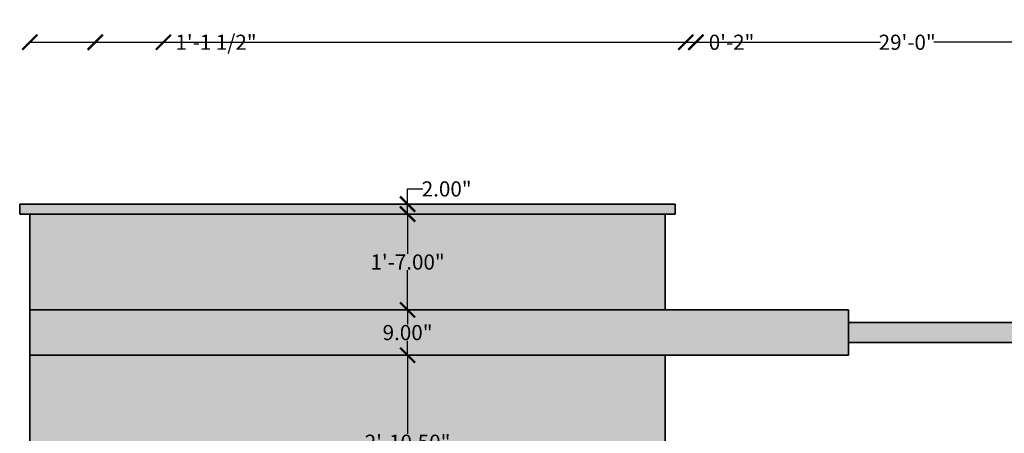
# Model space of a CAD drawing. Units: inches. Extents: x -654 to 390, y -40 to 648.
# Tile 12 of 13: x -3 to 192, y 566 to 648. Entities that reach past the tile are written whole.
import ezdxf

# ---------------------------------------------------------------- set-up
doc = ezdxf.new("R2010")
doc.units = ezdxf.units.IN
doc.header["$PDMODE"] = 3
for name, color, linetype, lineweight in [('A-ANNO-DIMS', 2, 'Continuous', 18), ('A-ELEV', 7, 'Continuous', 35), ('A-ELEV-FILL', 252, 'Continuous', 13)]:
    doc.layers.add(name, color=color, linetype=linetype, lineweight=lineweight)
doc.styles.get("Standard").update_dxf_attribs({"font": 'arial.ttf'})
doc.dimstyles.get("Standard").update_dxf_attribs({"dimtxt": 3, "dimasz": 3, "dimexe": 0.18, "dimexo": 0.0625, "dimgap": 0.09, "dimtad": 0, "dimtih": 1, "dimtoh": 1, "dimzin": 0, "dimdsep": 46, "dimlunit": 3, "dimtxsty": 'Standard', "dimblk": 'ARCHTICK', "dimcen": 0.09, "dimse1": 1, "dimse2": 1, "dimadec": 0, "dimazin": 0, "dimtfac": 1, "dimtofl": 0, "dimtmove": 0, "dimatfit": 3, "dimfxl": 1, "dimtolj": 1, "dimtzin": 0, "dimarcsym": 0})

# ---------------------------------------------------------------- blocks, each defined once
blk = doc.blocks.new('_ArchTick')
at = {"color": 0, "linetype": 'ByBlock', "const_width": 0.15}
blk.add_lwpolyline([(-0.5, -0.5), (0.5, 0.5)], dxfattribs=at)
blk = doc.blocks.new('*D8')
at = {"layer": 'A-ANNO-DIMS', "color": 0, "lineweight": -2, "transparency": 16777216}
for p, q in [((360.51, 590.13), (360.51, 545.26)), ((360.51, 497.13), (360.51, 542.01))]:
    blk.add_line(p, q, dxfattribs=at)
at = {"layer": 'Defpoints', "color": 0, "transparency": 16777216}
for p in [(161.04, 590.13), (360.51, 590.13), (346.65, 497.13)]:
    blk.add_point(p, dxfattribs=at)
at = {"layer": 'A-ANNO-DIMS', "color": 0, "lineweight": -2, "transparency": 16777216, "xscale": 3, "yscale": 3, "zscale": 3}
for p, rotation in [((360.51, 590.13), 90), ((360.51, 497.13), 270)]:
    blk.add_blockref('_ArchTick', p, dxfattribs=dict(at, rotation=rotation))
at = {"layer": 'A-ANNO-DIMS', "color": 0, "transparency": 16777216, "insert": (360.51, 543.63), "char_height": 3, "attachment_point": 5}
blk.add_mtext('\\A1;7\'-9.00"', dxfattribs=at)
blk = doc.blocks.new('*D9')
at = {"layer": 'A-ANNO-DIMS', "color": 0, "lineweight": -2, "transparency": 16777216}
for p, q in [((360.51, 611.13), (360.51, 602.26)), ((360.51, 590.13), (360.51, 599.01))]:
    blk.add_line(p, q, dxfattribs=at)
at = {"layer": 'Defpoints', "color": 0, "transparency": 16777216}
for p in [(126.65, 611.13), (360.51, 611.13), (161.04, 590.13)]:
    blk.add_point(p, dxfattribs=at)
at = {"layer": 'A-ANNO-DIMS', "color": 0, "lineweight": -2, "transparency": 16777216, "xscale": 3, "yscale": 3, "zscale": 3}
for p, rotation in [((360.51, 611.13), 90), ((360.51, 590.13), 270)]:
    blk.add_blockref('_ArchTick', p, dxfattribs=dict(at, rotation=rotation))
at = {"layer": 'A-ANNO-DIMS', "color": 0, "transparency": 16777216, "insert": (360.51, 600.63), "char_height": 3, "attachment_point": 5}
blk.add_mtext('\\A1;1\'-9.00"', dxfattribs=at)
blk = doc.blocks.new('*D10')
at = {"layer": 'A-ANNO-DIMS', "color": 0, "lineweight": -2, "transparency": 16777216}
for p, q in [((73.57, 611.13), (73.57, 614.13)), ((73.57, 614.13), (76.57, 614.13)), ((73.57, 609.13), (73.57, 611.13))]:
    blk.add_line(p, q, dxfattribs=at)
at = {"layer": 'Defpoints', "color": 0, "transparency": 16777216}
for p in [(61.65, 611.13), (73.57, 611.13), (61.65, 609.13)]:
    blk.add_point(p, dxfattribs=at)
at = {"layer": 'A-ANNO-DIMS', "color": 0, "lineweight": -2, "transparency": 16777216, "xscale": 3, "yscale": 3, "zscale": 3}
for p, rotation in [((73.57, 611.13), 90), ((73.57, 609.13), 270)]:
    blk.add_blockref('_ArchTick', p, dxfattribs=dict(at, rotation=rotation))
at = {"layer": 'A-ANNO-DIMS', "color": 0, "transparency": 16777216, "insert": (81.32, 614.13), "char_height": 3, "attachment_point": 5}
blk.add_mtext('\\A1;2.00"', dxfattribs=at)
blk = doc.blocks.new('*D11')
at = {"layer": 'A-ANNO-DIMS', "color": 0, "lineweight": -2, "transparency": 16777216}
for p, q in [((73.57, 609.13), (73.57, 601.26)), ((73.57, 590.13), (73.57, 598.01))]:
    blk.add_line(p, q, dxfattribs=at)
at = {"layer": 'Defpoints', "color": 0, "transparency": 16777216}
for p in [(73.57, 609.13), (73.57, 590.13), (73.57, 590.13)]:
    blk.add_point(p, dxfattribs=at)
at = {"layer": 'A-ANNO-DIMS', "color": 0, "lineweight": -2, "transparency": 16777216, "xscale": 3, "yscale": 3, "zscale": 3}
for p, rotation in [((73.57, 609.13), 90), ((73.57, 590.13), 270)]:
    blk.add_blockref('_ArchTick', p, dxfattribs=dict(at, rotation=rotation))
at = {"layer": 'A-ANNO-DIMS', "color": 0, "transparency": 16777216, "insert": (73.57, 599.63), "char_height": 3, "attachment_point": 5}
blk.add_mtext('\\A1;1\'-7.00"', dxfattribs=at)
blk = doc.blocks.new('*D12')
at = {"layer": 'A-ANNO-DIMS', "color": 0, "lineweight": -2, "transparency": 16777216}
for p, q in [((73.57, 590.13), (73.57, 587.26)), ((73.57, 581.13), (73.57, 584.01))]:
    blk.add_line(p, q, dxfattribs=at)
at = {"layer": 'Defpoints', "color": 0, "transparency": 16777216}
for p in [(73.57, 590.13), (73.57, 581.13), (73.57, 581.13)]:
    blk.add_point(p, dxfattribs=at)
at = {"layer": 'A-ANNO-DIMS', "color": 0, "lineweight": -2, "transparency": 16777216, "xscale": 3, "yscale": 3, "zscale": 3}
for p, rotation in [((73.57, 590.13), 90), ((73.57, 581.13), 270)]:
    blk.add_blockref('_ArchTick', p, dxfattribs=dict(at, rotation=rotation))
at = {"layer": 'A-ANNO-DIMS', "color": 0, "transparency": 16777216, "insert": (73.57, 585.63), "char_height": 3, "attachment_point": 5}
blk.add_mtext('\\A1;9.00"', dxfattribs=at)
blk = doc.blocks.new('*D13')
at = {"layer": 'A-ANNO-DIMS', "color": 0, "lineweight": -2, "transparency": 16777216}
for p, q in [((73.57, 581.13), (73.57, 565.51)), ((73.57, 546.63), (73.57, 562.26))]:
    blk.add_line(p, q, dxfattribs=at)
at = {"layer": 'Defpoints', "color": 0, "transparency": 16777216}
for p in [(73.57, 581.13), (57.15, 546.63), (73.57, 546.63)]:
    blk.add_point(p, dxfattribs=at)
at = {"layer": 'A-ANNO-DIMS', "color": 0, "lineweight": -2, "transparency": 16777216, "xscale": 3, "yscale": 3, "zscale": 3}
for p, rotation in [((73.57, 581.13), 90), ((73.57, 546.63), 270)]:
    blk.add_blockref('_ArchTick', p, dxfattribs=dict(at, rotation=rotation))
at = {"layer": 'A-ANNO-DIMS', "color": 0, "transparency": 16777216, "insert": (73.57, 563.88), "char_height": 3, "attachment_point": 5}
blk.add_mtext('\\A1;2\'-10.50"', dxfattribs=at)
blk = doc.blocks.new('*D75')
at = {"layer": 'A-ANNO-DIMS', "color": 0, "lineweight": -2, "transparency": 16777216}
for p, q in [((-1.35, 643.23), (167.38, 643.23)), ((346.65, 643.23), (177.91, 643.23))]:
    blk.add_line(p, q, dxfattribs=at)
at = {"layer": 'Defpoints', "color": 0, "transparency": 16777216}
for p in [(346.65, 643.23), (-1.35, 611.13), (346.65, 587.63)]:
    blk.add_point(p, dxfattribs=at)
at = {"layer": 'A-ANNO-DIMS', "color": 0, "lineweight": -2, "transparency": 16777216, "xscale": 3, "yscale": 3, "zscale": 3, "rotation": 180}
blk.add_blockref('_ArchTick', (-1.35, 643.23), dxfattribs=at)
at = {"layer": 'A-ANNO-DIMS', "color": 0, "lineweight": -2, "transparency": 16777216, "xscale": 3, "yscale": 3, "zscale": 3}
blk.add_blockref('_ArchTick', (346.65, 643.23), dxfattribs=at)
at = {"layer": 'A-ANNO-DIMS', "color": 0, "transparency": 16777216, "insert": (172.65, 643.23), "char_height": 3, "attachment_point": 5}
blk.add_mtext('\\A1;29\'-0"', dxfattribs=at)
blk = doc.blocks.new('*D76')
at = {"layer": 'A-ANNO-DIMS', "color": 0, "lineweight": -2, "transparency": 16777216}
for p, q in [((380.75, 611.13), (380.75, 306.76)), ((380.75, -0.87), (380.75, 303.51))]:
    blk.add_line(p, q, dxfattribs=at)
at = {"layer": 'Defpoints', "color": 0, "transparency": 16777216}
for p in [(126.65, 611.13), (380.75, 611.13), (346.65, -0.87)]:
    blk.add_point(p, dxfattribs=at)
at = {"layer": 'A-ANNO-DIMS', "color": 0, "lineweight": -2, "transparency": 16777216, "xscale": 3, "yscale": 3, "zscale": 3}
for p, rotation in [((380.75, 611.13), 90), ((380.75, -0.87), 270)]:
    blk.add_blockref('_ArchTick', p, dxfattribs=dict(at, rotation=rotation))
at = {"layer": 'A-ANNO-DIMS', "color": 0, "transparency": 16777216, "insert": (380.75, 305.13), "char_height": 3, "attachment_point": 5}
blk.add_mtext('\\A1;51\'-0"', dxfattribs=at)
blk = doc.blocks.new('*D80')
at = {"layer": 'A-ANNO-DIMS', "color": 0, "lineweight": -2, "transparency": 16777216}
for p, q in [((11.65, 643.23), (25.15, 643.23)), ((25.15, 643.23), (28.15, 643.23))]:
    blk.add_line(p, q, dxfattribs=at)
at = {"layer": 'Defpoints', "color": 0, "transparency": 16777216}
for p in [(25.15, 643.23), (11.65, 20.08), (25.15, 20.08)]:
    blk.add_point(p, dxfattribs=at)
at = {"layer": 'A-ANNO-DIMS', "color": 0, "lineweight": -2, "transparency": 16777216, "xscale": 3, "yscale": 3, "zscale": 3, "rotation": 180}
blk.add_blockref('_ArchTick', (11.65, 643.23), dxfattribs=at)
at = {"layer": 'A-ANNO-DIMS', "color": 0, "lineweight": -2, "transparency": 16777216, "xscale": 3, "yscale": 3, "zscale": 3}
blk.add_blockref('_ArchTick', (25.15, 643.23), dxfattribs=at)
at = {"layer": 'A-ANNO-DIMS', "color": 0, "transparency": 16777216, "insert": (35.58, 643.23), "char_height": 3, "attachment_point": 5}
blk.add_mtext('\\A1;1\'-1 1/2"', dxfattribs=at)
blk = doc.blocks.new('*D96')
at = {"layer": 'A-ANNO-DIMS', "color": 0, "lineweight": -2, "transparency": 16777216}
for p, q in [((128.74, 643.23), (130.74, 643.23)), ((130.74, 643.23), (133.74, 643.23))]:
    blk.add_line(p, q, dxfattribs=at)
at = {"layer": 'Defpoints', "color": 0, "transparency": 16777216}
for p in [(130.74, 643.23), (128.74, 311.13), (130.74, 311.13)]:
    blk.add_point(p, dxfattribs=at)
at = {"layer": 'A-ANNO-DIMS', "color": 0, "lineweight": -2, "transparency": 16777216, "xscale": 3, "yscale": 3, "zscale": 3, "rotation": 180}
blk.add_blockref('_ArchTick', (128.74, 643.23), dxfattribs=at)
at = {"layer": 'A-ANNO-DIMS', "color": 0, "lineweight": -2, "transparency": 16777216, "xscale": 3, "yscale": 3, "zscale": 3}
blk.add_blockref('_ArchTick', (130.74, 643.23), dxfattribs=at)
at = {"layer": 'A-ANNO-DIMS', "color": 0, "transparency": 16777216, "insert": (137.82, 643.23), "char_height": 3, "attachment_point": 5}
blk.add_mtext('\\A1;0\'-2"', dxfattribs=at)

msp = doc.modelspace()

# ---------------------------------------------------------------- hatches: boundary and pattern name
at = {"layer": 'A-ELEV-FILL'}
h = msp.add_hatch(color=256, dxfattribs=at)
h.dxf.hatch_style = 1
h.paths.add_polyline_path([(126.646, 611.134), (124.646, 611.134), (-1.354, 611.134), (-3.354, 611.134), (-3.354, 609.134), (-1.354, 609.134), (124.646, 609.134), (126.646, 609.134)])
h.paths.add_polyline_path([(8.646, 497.134), (-2.354, 497.134), (-2.354, 495.134), (8.646, 495.134)])
h.paths.add_polyline_path([(346.646, 497.134), (182.515, 497.134), (182.515, 495.134), (346.646, 495.134)])
h.paths.add_polyline_path([(198.646, 486.134), (198.646, 473.634), (209.366, 474.634), (199.646, 474.634), (199.646, 485.134), (209.366, 485.134)])
h.paths.add_polyline_path([(332.646, 486.134), (198.646, 486.134), (209.366, 485.134), (321.926, 485.134)])
h.paths.add_polyline_path([(321.926, 474.634), (209.366, 474.634), (198.646, 473.634), (332.646, 473.634)])
h.paths.add_polyline_path([(332.646, 486.134), (321.926, 485.134), (331.646, 485.134), (331.646, 474.634), (321.926, 474.634), (332.646, 473.634)])
h = msp.add_hatch(color=256, dxfattribs=at)
h.dxf.hatch_style = 1
h.paths.add_polyline_path([(115.646, 305.634), (97.646, 305.634), (97.646, 306.634), (98.293, 306.634), (98.293, 315.634), (97.646, 315.634), (97.646, 316.634), (100.646, 316.634), (100.646, 442.634), (-1.354, 442.634), (-1.354, 125.134), (115.646, 125.134)])
h.paths.add_polyline_path([(57.146, 161.134), (12.146, 161.134), (12.146, 413.134), (57.146, 413.134)], flags=16)
h.paths.add_polyline_path([(52.646, 165.634), (16.646, 165.634), (16.646, 408.634), (52.646, 408.634)], flags=0)
h.paths.add_polyline_path([(52.146, 166.134), (17.146, 166.134), (17.146, 408.134), (52.146, 408.134)], flags=0)
h.paths.add_polyline_path([(124.646, 581.134), (-1.354, 581.134), (-1.354, 497.134), (8.646, 497.134), (8.646, 494.634), (12.146, 494.634), (12.146, 546.634), (57.146, 546.634), (57.146, 494.634), (124.646, 494.634)])
h.paths.add_polyline_path([(124.646, 609.134), (-1.354, 609.134), (-1.354, 590.134), (124.646, 590.134)])
h = msp.add_hatch(color=256, dxfattribs=at)
h.dxf.hatch_style = 1
h.paths.add_polyline_path([(161.035, 590.134), (-1.354, 590.134), (-1.354, 581.134), (161.035, 581.134)])
h.paths.add_polyline_path([(346.646, 453.634), (-1.354, 453.634), (-1.354, 444.634), (337.646, 444.634), (337.646, 177.634), (178.742, 177.634), (178.742, 173.134), (176.742, 173.134), (176.742, 177.634), (166.742, 177.634), (166.742, 173.134), (164.742, 173.134), (164.742, 177.634), (154.742, 177.634), (154.742, 173.134), (152.742, 173.134), (152.742, 177.634), (142.742, 177.634), (142.742, 173.134), (140.742, 173.134), (140.742, 177.634), (130.742, 177.634), (130.742, 173.134), (128.742, 173.134), (128.742, 177.634), (115.646, 177.634), (115.646, 168.634), (346.646, 168.634), (346.646, 173.134)])
h.paths.add_polyline_path([(7.646, 87.642), (-1.354, 87.642), (-1.354, 17.134), (7.646, 17.134)])
h.paths.add_polyline_path([(16.396, 116.134), (60.646, 116.134), (60.646, 83.134), (62.646, 83.134), (113.646, 83.134), (115.646, 83.134), (115.646, 125.134), (7.646, 125.134), (7.646, 89.642), (8.146, 89.642), (8.146, 87.642), (7.646, 87.642), (7.646, 83.134), (9.646, 83.134), (16.396, 83.134)])
h = msp.add_hatch(color=256, dxfattribs=at)
h.dxf.hatch_style = 1
h.paths.add_polyline_path([(346.646, 587.634), (161.035, 587.634), (161.035, 583.634), (342.646, 583.634), (342.646, 497.134), (346.646, 497.134), (346.646, 583.634)])
h.paths.add_polyline_path([(295.646, 315.634), (98.293, 315.634), (98.293, 311.134), (295.646, 311.134)])
h.paths.add_polyline_path([(128.742, 311.134), (98.293, 311.134), (98.293, 306.634), (128.742, 306.634)])
h.paths.add_polyline_path([(140.742, 311.134), (130.742, 311.134), (130.742, 306.634), (140.742, 306.634)])
h.paths.add_polyline_path([(152.742, 311.134), (142.742, 311.134), (142.742, 306.634), (152.742, 306.634)])
h.paths.add_polyline_path([(164.742, 311.134), (154.742, 311.134), (154.742, 306.634), (164.742, 306.634)])
h.paths.add_polyline_path([(176.742, 311.134), (166.742, 311.134), (166.742, 306.634), (176.742, 306.634)])
h.paths.add_polyline_path([(295.646, 311.134), (178.742, 311.134), (178.742, 306.634), (295.646, 306.634)])
h.paths.add_polyline_path([(303.818, 315.634), (295.646, 315.634), (295.646, 311.134), (303.818, 311.134)])
h.paths.add_polyline_path([(303.818, 311.134), (295.646, 311.134), (295.646, 306.634), (303.818, 306.634)])

# ---------------------------------------------------------------- linework, layer by layer
at = {"layer": 'A-ELEV'}
for p, q in [((-3.354, 609.134), (-3.354, 611.134)), ((-3.354, 611.134), (-1.354, 611.134)), ((-1.354, 611.134), (124.646, 611.134)), ((126.646, 611.134), (124.646, 611.134)), ((126.646, 609.134), (126.646, 611.134)), ((-1.354, 609.134), (-3.354, 609.134)), ((-1.354, 497.134), (-1.354, 609.134)), ((-1.354, 609.134), (124.646, 609.134)), ((124.646, 609.134), (124.646, 590.134)), ((124.646, 609.134), (126.646, 609.134)), ((-1.354, 590.134), (161.035, 590.134)), ((161.035, 590.134), (161.035, 581.134)), ((161.035, 587.634), (346.646, 587.634)), ((161.035, 583.634), (342.646, 583.634)), ((-1.354, 581.134), (161.035, 581.134)), ((124.646, 581.134), (124.646, 494.634))]:
    msp.add_line(p, q, dxfattribs=at)

# ---------------------------------------------------------------- dimensions: what is measured, and where the dimension line sits
at = {"layer": 'A-ANNO-DIMS'}
for base, p1, p2, picture, middle in [((25.146, 643.234), (11.646, 20.08), (25.146, 20.08), '*D80', (35.578, 643.234)), ((346.646, 643.234), (-1.354, 611.134), (346.646, 587.634), '*D75', (172.646, 643.234)), ((130.742, 643.234), (128.742, 311.134), (130.742, 311.134), '*D96', (137.82, 643.234))]:
    dim = msp.add_linear_dim(base=base, p1=p1, p2=p2, dimstyle='Standard', override={"dimdec": 1, "dimlfac": 1, "dimrnd": 0, "dimzin": 1, "dimdsep": 46, "dimlunit": 4, "dimfrac": 2}, dxfattribs=at)
    dim.commit()
    dim.dimension.update_dxf_attribs({"geometry": picture, "text_midpoint": middle})
for base, p1, p2, override, picture, middle in [((73.566, 611.134), (61.646, 609.134), (61.646, 611.134), {"dimclrd": 0, "dimclre": 0, "dimclrt": 0}, '*D10', (81.319, 614.134)), ((360.508, 611.134), (161.035, 590.134), (126.646, 611.134), {"dimclrd": 0, "dimclre": 0, "dimclrt": 0, "dimtmove": 1}, '*D9', (360.508, 600.634)), ((380.746, 611.134), (346.646, -0.866), (126.646, 611.134), {"dimdec": 1, "dimlfac": 1, "dimrnd": 0, "dimzin": 1, "dimdsep": 46, "dimlunit": 4, "dimfrac": 2}, '*D76', (380.746, 305.134)), ((73.566, 590.134), (73.566, 609.134), (73.566, 590.134), {"dimclrd": 0, "dimclre": 0, "dimclrt": 0}, '*D11', (73.566, 599.634)), ((73.566, 581.134), (73.566, 590.134), (73.566, 581.134), {"dimclrd": 0, "dimclre": 0, "dimclrt": 0, "dimtmove": 1}, '*D12', (73.566, 585.634)), ((360.508, 590.134), (346.646, 497.134), (161.035, 590.134), {"dimclrd": 0, "dimclre": 0, "dimclrt": 0, "dimtmove": 1}, '*D8', (360.508, 543.634)), ((73.566, 546.634), (73.566, 581.134), (57.146, 546.634), {"dimclrd": 0, "dimclre": 0, "dimclrt": 0, "dimtmove": 1}, '*D13', (73.566, 563.884))]:
    dim = msp.add_linear_dim(base=base, p1=p1, p2=p2, angle=90, dimstyle='Standard', override=override, dxfattribs=at)
    dim.commit()
    dim.dimension.update_dxf_attribs({"geometry": picture, "text_midpoint": middle})

doc.saveas('drawing.dxf')
